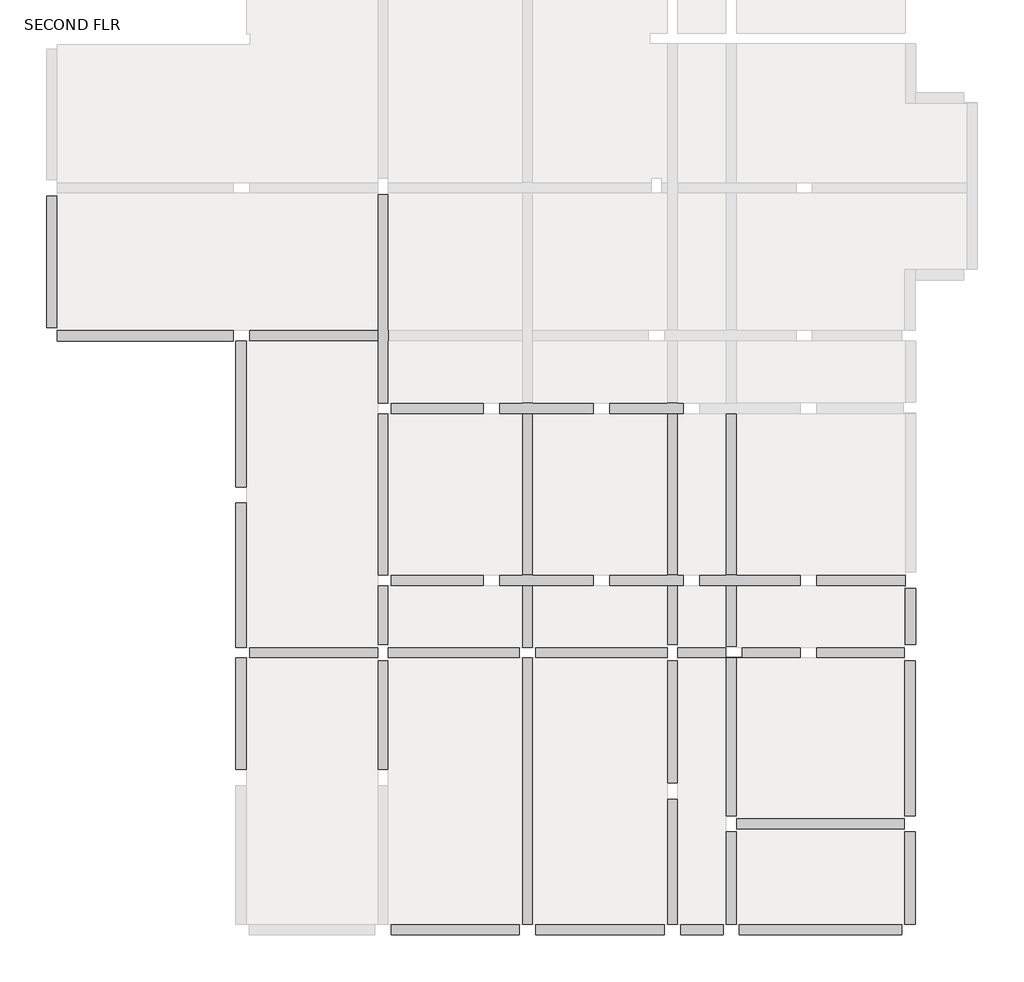
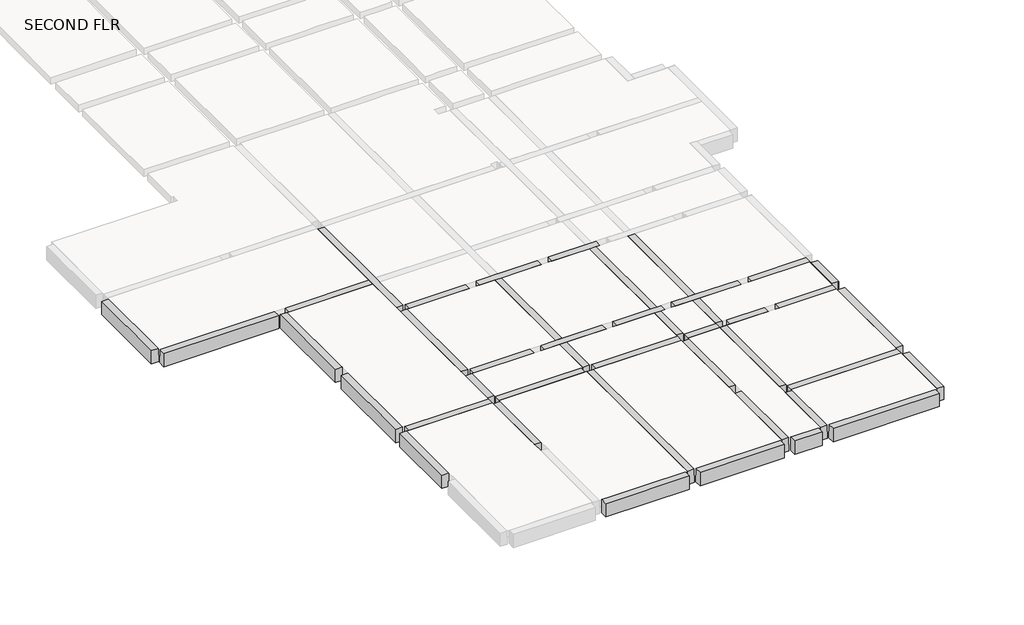
# One storey, part 2 of 4: 42 beams.
"""IFC4 building model written with IfcOpenShell, lengths in millimetres."""

from ifc_helpers import new_model, si_unit, frame, origin, place, context, project, spatial, polyline, outline, extrude, faceted_brep, element, save

model = new_model("IFC4")

# Units and contexts
model_context = context("Model", 3, world=origin())
ifc_project = project(units=[si_unit("LENGTHUNIT", "METRE", prefix="MILLI")], contexts=[model_context])

# Site, building, storey
site = spatial("IfcSite", under=ifc_project)
building = spatial("IfcBuilding", under=site)
storey = spatial("IfcBuildingStorey", under=building, Name="SECOND FLR", Elevation=6048.0)

# Beams
placement = place(None, origin())
element("IfcBeam", 1, ObjectType="M_Concrete-Rectangular Beam : 300 x 600mm", at=placement, inside=storey, context=model_context, shape_type="SweptSolid", body=[
    extrude(outline(polyline([(-10828.8105653, -2764.4535766), (-11128.8105653, -2764.4535766), (-11128.8105653, 876.1713929), (-10828.8105653, 876.1713929), (-10828.8105653, -2764.4535766)])), frame((0.0, 0.0, 5448.0), z_axis=(0.0, 0.0, 1.0), x_axis=(1.0, 0.0, 0.0)), (0.0, 0.0, 1.0), 600.0),
])
element("IfcBeam", 2, ObjectType="M_Concrete-Rectangular Beam : 300 x 600mm", at=placement, inside=storey, context=model_context, shape_type="Brep", body=[
    faceted_brep([(-5963.8105653, -3139.4535766, 6048.0), (-5963.8105653, -2839.4535766, 6048.0), (-10828.8105653, -2839.4535766, 6048.0), (-10828.8105653, -3139.4535766, 6048.0), (-5963.8105653, -3139.4535766, 5448.0), (-10828.8105653, -3139.4535766, 5448.0), (-5963.8105653, -2839.4535766, 5448.0), (-10828.8105653, -2839.4535766, 5448.0), (-5963.8105653, -2839.4535766, 5748.0), (-10828.8105653, -2839.4535766, 5748.0)], [[[0, 1, 2, 3]], [[4, 0, 3, 5]], [[6, 4, 5, 7]], [[2, 1, 8, 6, 7, 9]], [[1, 0, 4, 6, 8]], [[3, 2, 9, 7, 5]]]),
])
element("IfcBeam", 3, ObjectType="M_Concrete-Rectangular Beam : 300 x 600mm", at=placement, inside=storey, context=model_context, shape_type="Brep", body=[
    faceted_brep([(-5588.8105653, -7169.0760584, 6048.0), (-5588.8105653, -3139.4535766, 6048.0), (-5888.8105653, -3139.4535766, 6048.0), (-5888.8105653, -7169.0760584, 6048.0), (-5888.8105653, -3139.4535766, 5448.0), (-5888.8105653, -7169.0760584, 5448.0), (-5588.8105653, -3139.4535766, 5448.0), (-5588.8105653, -7169.0760584, 5448.0), (-5588.8105653, -7169.0760584, 5748.0), (-5588.8105653, -3139.4535766, 5748.0)], [[[0, 1, 2, 3]], [[3, 2, 4, 5]], [[5, 4, 6, 7]], [[1, 0, 8, 7, 6, 9]], [[6, 4, 2, 1, 9]], [[0, 3, 5, 7, 8]]]),
])
element("IfcBeam", 4, ObjectType="M_Concrete-Rectangular Beam : 300 x 600mm", at=placement, inside=storey, context=model_context, shape_type="Brep", body=[
    faceted_brep([(-5588.8105653, -11607.8970059, 6048.0), (-5588.8105653, -7619.0760584, 6048.0), (-5888.8105653, -7619.0760584, 6048.0), (-5888.8105653, -11607.8970059, 6048.0), (-5888.8105653, -7619.0760584, 5448.0), (-5888.8105653, -11607.8970059, 5448.0), (-5588.8105653, -7619.0760584, 5448.0), (-5588.8105653, -11607.8970059, 5448.0), (-5588.8105653, -11607.8970059, 5748.0), (-5588.8105653, -7619.0760584, 5748.0)], [[[0, 1, 2, 3]], [[3, 2, 4, 5]], [[5, 4, 6, 7]], [[1, 0, 8, 7, 6, 9]], [[0, 3, 5, 7, 8]], [[6, 4, 2, 1, 9]]]),
])
element("IfcBeam", 5, ObjectType="M_Concrete-Rectangular Beam : 300 x 600mm", at=placement, inside=storey, context=model_context, shape_type="Brep", body=[
    faceted_brep([(-5588.8105653, -14991.2517597, 6048.0), (-5588.8105653, -11907.8970059, 6048.0), (-5888.8105653, -11907.8970059, 6048.0), (-5888.8105653, -14991.2517597, 6048.0), (-5888.8105653, -11907.8970059, 5448.0), (-5888.8105653, -14991.2517597, 5448.0), (-5588.8105653, -11907.8970059, 5448.0), (-5588.8105653, -14991.2517597, 5448.0), (-5588.8105653, -14991.2517597, 5748.0), (-5588.8105653, -11907.8970059, 5748.0)], [[[0, 1, 2, 3]], [[3, 2, 4, 5]], [[5, 4, 6, 7]], [[1, 0, 8, 7, 6, 9]], [[6, 4, 2, 1, 9]], [[0, 3, 5, 7, 8]]]),
])
element("IfcBeam", 6, ObjectType="M_Concrete-Rectangular Beam : 300 x 600mm", at=placement, inside=storey, context=model_context, shape_type="SweptSolid", body=[
    extrude(outline(polyline([(1949.7296816, -19272.5304373), (1949.7296816, -19572.5304373), (-1596.7865686, -19572.5304373), (-1596.7865686, -19272.5304373), (1949.7296816, -19272.5304373)])), frame((0.0, 0.0, 5448.0), z_axis=(0.0, 0.0, 1.0), x_axis=(1.0, 0.0, 0.0)), (0.0, 0.0, 1.0), 600.0),
])
element("IfcBeam", 7, ObjectType="M_Concrete-Rectangular Beam : 300 x 600mm", at=placement, inside=storey, context=model_context, shape_type="SweptSolid", body=[
    extrude(outline(polyline([(5957.5248054, -19272.5304373), (5957.5248054, -19572.5304373), (2399.7296816, -19572.5304373), (2399.7296816, -19272.5304373), (5957.5248054, -19272.5304373)])), frame((0.0, 0.0, 5448.0), z_axis=(0.0, 0.0, 1.0), x_axis=(1.0, 0.0, 0.0)), (0.0, 0.0, 1.0), 600.0),
])
element("IfcBeam", 8, ObjectType="M_Concrete-Rectangular Beam : 300 x 600mm", at=placement, inside=storey, context=model_context, shape_type="SweptSolid", body=[
    extrude(outline(polyline([(7581.8679014, -19272.5304373), (7581.8679014, -19572.5304373), (6407.5248054, -19572.5304373), (6407.5248054, -19272.5304373), (7581.8679014, -19272.5304373)])), frame((0.0, 0.0, 5448.0), z_axis=(0.0, 0.0, 1.0), x_axis=(1.0, 0.0, 0.0)), (0.0, 0.0, 1.0), 600.0),
])
element("IfcBeam", 9, ObjectType="M_Concrete-Rectangular Beam : 300 x 600mm", at=placement, inside=storey, context=model_context, shape_type="SweptSolid", body=[
    extrude(outline(polyline([(12524.1163908, -19272.5304373), (12524.1163908, -19572.5304373), (8031.8679014, -19572.5304373), (8031.8679014, -19272.5304373), (12524.1163908, -19272.5304373)])), frame((0.0, 0.0, 5448.0), z_axis=(0.0, 0.0, 1.0), x_axis=(1.0, 0.0, 0.0)), (0.0, 0.0, 1.0), 600.0),
])
element("IfcBeam", 10, ObjectType="M_Concrete-Rectangular Beam : 300 x 600mm", at=placement, inside=storey, context=model_context, shape_type="Brep", body=[
    faceted_brep([(12599.1163908, -19272.5304373, 6048.0), (12899.1163908, -19272.5304373, 6048.0), (12899.1163908, -16719.1579597, 6048.0), (12599.1163908, -16719.1579597, 6048.0), (12899.1163908, -19272.5304373, 5448.0), (12899.1163908, -16719.1579597, 5448.0), (12599.1163908, -19272.5304373, 5448.0), (12599.1163908, -16719.1579597, 5448.0), (12599.1163908, -16719.1579597, 5748.0), (12599.1163908, -19272.5304373, 5748.0)], [[[0, 1, 2, 3]], [[1, 4, 5, 2]], [[4, 6, 7, 5]], [[0, 3, 8, 7, 6, 9]], [[6, 4, 1, 0, 9]], [[3, 2, 5, 7, 8]]]),
])
element("IfcBeam", 11, ObjectType="M_Concrete-Rectangular Beam : 300 x 600mm", at=placement, inside=storey, context=model_context, shape_type="Brep", body=[
    faceted_brep([(12599.1163908, -16269.1579597, 6048.0), (12899.1163908, -16269.1579597, 6048.0), (12899.1163908, -11982.8970059, 6048.0), (12599.1163908, -11982.8970059, 6048.0), (12899.1163908, -16269.1579597, 5448.0), (12899.1163908, -11982.8970059, 5448.0), (12599.1163908, -16269.1579597, 5448.0), (12599.1163908, -11982.8970059, 5448.0), (12599.1163908, -11982.8970059, 5748.0), (12599.1163908, -16269.1579597, 5748.0)], [[[0, 1, 2, 3]], [[1, 4, 5, 2]], [[4, 6, 7, 5]], [[0, 3, 8, 7, 6, 9]], [[6, 4, 1, 0, 9]], [[3, 2, 5, 7, 8]]]),
])
element("IfcBeam", 12, ObjectType="M_Concrete-Rectangular Beam : 300 x 600mm", at=placement, inside=storey, context=model_context, shape_type="SweptSolid", body=[
    extrude(outline(polyline([(12619.1163908, -9982.1078267), (12919.1163908, -9982.1078267), (12919.1163908, -11537.8970059), (12899.1163908, -11537.8970059), (12899.1163908, -11532.8970059), (12619.1163908, -11532.8970059), (12619.1163908, -9982.1078267)])), frame((0.0, 0.0, 5448.0), z_axis=(0.0, 0.0, 1.0), x_axis=(1.0, 0.0, 0.0)), (0.0, 0.0, 1.0), 600.0),
])
element("IfcBeam", 13, ObjectType="M_Concrete-Rectangular Beam : 300 x 600mm", at=placement, inside=storey, context=model_context, shape_type="Brep", body=[
    faceted_brep([(-1971.7865686, -11982.8970059, 6048.0), (-1971.7865686, -14991.2517597, 6048.0), (-1671.7865686, -14991.2517597, 6048.0), (-1671.7865686, -11982.8970059, 6048.0), (-1671.7865686, -14991.2517597, 5748.0), (-1671.7865686, -14991.2517597, 5448.0), (-1671.7865686, -11982.8970059, 5448.0), (-1671.7865686, -11982.8970059, 5748.0), (-1971.7865686, -14991.2517597, 5448.0), (-1971.7865686, -11982.8970059, 5448.0), (-1971.7865686, -11982.8970059, 5748.0), (-1971.7865686, -14991.2517597, 5748.0)], [[[0, 1, 2, 3]], [[3, 2, 4, 5, 6, 7]], [[6, 5, 8, 9]], [[1, 0, 10, 9, 8, 11]], [[0, 3, 7, 6, 9, 10]], [[8, 5, 4, 2, 1, 11]]]),
])
element("IfcBeam", 14, ObjectType="M_Concrete-Rectangular Beam : 300 x 600mm", at=placement, inside=storey, context=model_context, shape_type="Brep", body=[
    faceted_brep([(-1971.7865686, -9907.1078267, 6048.0), (-1971.7865686, -11532.8970059, 6048.0), (-1671.7865686, -11532.8970059, 6048.0), (-1671.7865686, -9907.1078267, 6048.0), (-1671.7865686, -11532.8970059, 5748.0), (-1671.7865686, -11532.8970059, 5448.0), (-1671.7865686, -9907.1078267, 5448.0), (-1671.7865686, -9907.1078267, 5748.0), (-1971.7865686, -11532.8970059, 5448.0), (-1971.7865686, -9907.1078267, 5448.0), (-1971.7865686, -9907.1078267, 5748.0), (-1971.7865686, -11532.8970059, 5748.0)], [[[0, 1, 2, 3]], [[3, 2, 4, 5, 6, 7]], [[6, 5, 8, 9]], [[1, 0, 10, 9, 8, 11]], [[0, 3, 7, 6, 9, 10]], [[8, 5, 4, 2, 1, 11]]]),
])
element("IfcBeam", 15, ObjectType="M_Concrete-Rectangular Beam : 300 x 600mm", at=placement, inside=storey, context=model_context, shape_type="Brep", body=[
    faceted_brep([(-1671.7865686, 916.1713929, 6048.0), (-1971.7865686, 916.1713929, 6048.0), (-1971.7865686, -2839.4535766, 6048.0), (-1971.7865686, -3139.4535766, 6048.0), (-1971.7865686, -4851.6229916, 6048.0), (-1671.7865686, -4851.6229916, 6048.0), (-1671.7865686, -3139.4535766, 6048.0), (-1671.7865686, -2839.4535766, 6048.0), (-1971.7865686, 916.1713929, 5448.0), (-1971.7865686, -2839.4535766, 5448.0), (-1971.7865686, -3139.4535766, 5448.0), (-1971.7865686, -4851.6229916, 5448.0), (-1971.7865686, -4851.6229916, 5748.0), (-1971.7865686, 916.1713929, 5748.0), (-1671.7865686, 916.1713929, 5448.0), (-1671.7865686, -2839.4535766, 5448.0), (-1671.7865686, -3139.4535766, 5448.0), (-1671.7865686, -4851.6229916, 5448.0), (-1671.7865686, 916.1713929, 5748.0), (-1671.7865686, -4851.6229916, 5748.0)], [[[0, 1, 2, 3, 4, 5, 6, 7]], [[8, 9, 10, 11, 12, 4, 3, 2, 1, 13]], [[8, 14, 15, 16, 17, 11, 10, 9]], [[17, 16, 15, 14, 18, 0, 7, 6, 5, 19]], [[1, 0, 18, 14, 8, 13]], [[5, 4, 12, 11, 17, 19]]]),
])
element("IfcBeam", 16, ObjectType="M_Concrete-Rectangular Beam : 300 x 600mm", at=placement, inside=storey, context=model_context, shape_type="Brep", body=[
    faceted_brep([(-1671.7865686, -5151.6229916, 6048.0), (-1971.7865686, -5151.6229916, 6048.0), (-1971.7865686, -9607.1078267, 6048.0), (-1671.7865686, -9607.1078267, 6048.0), (-1971.7865686, -5151.6229916, 5748.0), (-1971.7865686, -5151.6229916, 5448.0), (-1971.7865686, -9607.1078267, 5448.0), (-1971.7865686, -9607.1078267, 5748.0), (-1671.7865686, -5151.6229916, 5448.0), (-1671.7865686, -9607.1078267, 5448.0), (-1671.7865686, -9607.1078267, 5748.0), (-1671.7865686, -5151.6229916, 5748.0)], [[[0, 1, 2, 3]], [[2, 1, 4, 5, 6, 7]], [[5, 8, 9, 6]], [[0, 3, 10, 9, 8, 11]], [[1, 0, 11, 8, 5, 4]], [[3, 2, 7, 6, 9, 10]]]),
])
element("IfcBeam", 17, ObjectType="M_Concrete-Rectangular Beam : 300 x 600mm", at=placement, inside=storey, context=model_context, shape_type="Brep", body=[
    faceted_brep([(2324.7296816, -11907.8970059, 6048.0), (2024.7296816, -11907.8970059, 6048.0), (2024.7296816, -19272.5304373, 6048.0), (2324.7296816, -19272.5304373, 6048.0), (2024.7296816, -11907.8970059, 5748.0), (2024.7296816, -11907.8970059, 5448.0), (2024.7296816, -19272.5304373, 5448.0), (2024.7296816, -19272.5304373, 5748.0), (2324.7296816, -11907.8970059, 5448.0), (2324.7296816, -19272.5304373, 5448.0), (2324.7296816, -19272.5304373, 5748.0), (2324.7296816, -11907.8970059, 5748.0)], [[[0, 1, 2, 3]], [[2, 1, 4, 5, 6, 7]], [[5, 8, 9, 6]], [[0, 3, 10, 9, 8, 11]], [[1, 0, 11, 8, 5, 4]], [[3, 2, 7, 6, 9, 10]]]),
])
element("IfcBeam", 18, ObjectType="M_Concrete-Rectangular Beam : 300 x 600mm", at=placement, inside=storey, context=model_context, shape_type="Brep", body=[
    faceted_brep([(6332.5248054, -11982.8970059, 6048.0), (6032.5248054, -11982.8970059, 6048.0), (6032.5248054, -15369.1579597, 6048.0), (6332.5248054, -15369.1579597, 6048.0), (6032.5248054, -11982.8970059, 5748.0), (6032.5248054, -11982.8970059, 5448.0), (6032.5248054, -15369.1579597, 5448.0), (6032.5248054, -15369.1579597, 5748.0), (6332.5248054, -11982.8970059, 5448.0), (6332.5248054, -15369.1579597, 5448.0), (6332.5248054, -15369.1579597, 5748.0), (6332.5248054, -11982.8970059, 5748.0)], [[[0, 1, 2, 3]], [[2, 1, 4, 5, 6, 7]], [[5, 8, 9, 6]], [[0, 3, 10, 9, 8, 11]], [[1, 0, 11, 8, 5, 4]], [[3, 2, 7, 6, 9, 10]]]),
])
element("IfcBeam", 19, ObjectType="M_Concrete-Rectangular Beam : 300 x 600mm", at=placement, inside=storey, context=model_context, shape_type="Brep", body=[
    faceted_brep([(6032.5248054, -19272.5304373, 6048.0), (6332.5248054, -19272.5304373, 6048.0), (6332.5248054, -15819.1579597, 6048.0), (6032.5248054, -15819.1579597, 6048.0), (6032.5248054, -15819.1579597, 5748.0), (6032.5248054, -15819.1579597, 5448.0), (6032.5248054, -19272.5304373, 5448.0), (6032.5248054, -19272.5304373, 5748.0), (6332.5248054, -19272.5304373, 5448.0), (6332.5248054, -15819.1579597, 5448.0), (6332.5248054, -19272.5304373, 5748.0), (6332.5248054, -15819.1579597, 5748.0)], [[[0, 1, 2, 3]], [[0, 3, 4, 5, 6, 7]], [[8, 6, 5, 9]], [[2, 1, 10, 8, 9, 11]], [[1, 0, 7, 6, 8, 10]], [[3, 2, 11, 9, 5, 4]]]),
])
element("IfcBeam", 20, ObjectType="M_Concrete-Rectangular Beam : 300 x 600mm", at=placement, inside=storey, context=model_context, shape_type="Brep", body=[
    faceted_brep([(7656.8679014, -19272.5304373, 6048.0), (7956.8679014, -19272.5304373, 6048.0), (7956.8679014, -16719.1579597, 6048.0), (7656.8679014, -16719.1579597, 6048.0), (7656.8679014, -16719.1579597, 5748.0), (7656.8679014, -16719.1579597, 5448.0), (7656.8679014, -19272.5304373, 5448.0), (7656.8679014, -19272.5304373, 5748.0), (7956.8679014, -19272.5304373, 5448.0), (7956.8679014, -16719.1579597, 5448.0), (7956.8679014, -19272.5304373, 5748.0), (7956.8679014, -16719.1579597, 5748.0)], [[[0, 1, 2, 3]], [[0, 3, 4, 5, 6, 7]], [[8, 6, 5, 9]], [[2, 1, 10, 8, 9, 11]], [[1, 0, 7, 6, 8, 10]], [[3, 2, 11, 9, 5, 4]]]),
])
element("IfcBeam", 21, ObjectType="M_Concrete-Rectangular Beam : 300 x 600mm", at=placement, inside=storey, context=model_context, shape_type="Brep", body=[
    faceted_brep([(-5513.8105653, -2839.4535766, 6048.0), (-5513.8105653, -3139.4535766, 6048.0), (-1971.7865686, -3139.4535766, 6048.0), (-1971.7865686, -2839.4535766, 6048.0), (-5513.8105653, -3139.4535766, 5748.0), (-5513.8105653, -3139.4535766, 5448.0), (-1971.7865686, -3139.4535766, 5448.0), (-1971.7865686, -3139.4535766, 5748.0), (-5513.8105653, -2839.4535766, 5448.0), (-1971.7865686, -2839.4535766, 5448.0), (-1971.7865686, -2839.4535766, 5748.0), (-5513.8105653, -2839.4535766, 5748.0)], [[[0, 1, 2, 3]], [[2, 1, 4, 5, 6, 7]], [[5, 8, 9, 6]], [[0, 3, 10, 9, 8, 11]], [[1, 0, 11, 8, 5, 4]], [[3, 2, 7, 6, 9, 10]]]),
])
element("IfcBeam", 22, ObjectType="M_Concrete-Rectangular Beam : 300 x 600mm", at=placement, inside=storey, context=model_context, shape_type="Brep", body=[
    faceted_brep([(-1596.7865686, -4851.6229916, 6048.0), (-1596.7865686, -5151.6229916, 6048.0), (949.7296816, -5151.6229916, 6048.0), (949.7296816, -4851.6229916, 6048.0), (-1596.7865686, -5151.6229916, 5748.0), (-1596.7865686, -5151.6229916, 5448.0), (949.7296816, -5151.6229916, 5448.0), (949.7296816, -5151.6229916, 5748.0), (-1596.7865686, -4851.6229916, 5448.0), (949.7296816, -4851.6229916, 5448.0), (949.7296816, -4851.6229916, 5748.0), (-1596.7865686, -4851.6229916, 5748.0)], [[[0, 1, 2, 3]], [[2, 1, 4, 5, 6, 7]], [[5, 8, 9, 6]], [[0, 3, 10, 9, 8, 11]], [[1, 0, 11, 8, 5, 4]], [[3, 2, 7, 6, 9, 10]]]),
])
element("IfcBeam", 23, ObjectType="M_Concrete-Rectangular Beam : 300 x 600mm", at=placement, inside=storey, context=model_context, shape_type="Brep", body=[
    faceted_brep([(1399.7296816, -4851.6229916, 6048.0), (1399.7296816, -5151.6229916, 6048.0), (2024.7296816, -5151.6229916, 6048.0), (2324.7296816, -5151.6229916, 6048.0), (3997.5248054, -5151.6229916, 6048.0), (3997.5248054, -4851.6229916, 6048.0), (2324.7296816, -4851.6229916, 6048.0), (2024.7296816, -4851.6229916, 6048.0), (1399.7296816, -5151.6229916, 5448.0), (2024.7296816, -5151.6229916, 5448.0), (2324.7296816, -5151.6229916, 5448.0), (3997.5248054, -5151.6229916, 5448.0), (3997.5248054, -5151.6229916, 5748.0), (1399.7296816, -5151.6229916, 5748.0), (1399.7296816, -4851.6229916, 5448.0), (2024.7296816, -4851.6229916, 5448.0), (2324.7296816, -4851.6229916, 5448.0), (3997.5248054, -4851.6229916, 5448.0), (1399.7296816, -4851.6229916, 5748.0), (3997.5248054, -4851.6229916, 5748.0)], [[[0, 1, 2, 3, 4, 5, 6, 7]], [[8, 9, 10, 11, 12, 4, 3, 2, 1, 13]], [[8, 14, 15, 16, 17, 11, 10, 9]], [[17, 16, 15, 14, 18, 0, 7, 6, 5, 19]], [[1, 0, 18, 14, 8, 13]], [[5, 4, 12, 11, 17, 19]]]),
])
element("IfcBeam", 24, ObjectType="M_Concrete-Rectangular Beam : 300 x 600mm", at=placement, inside=storey, context=model_context, shape_type="Brep", body=[
    faceted_brep([(4447.5248054, -4851.6229916, 6048.0), (4447.5248054, -5151.6229916, 6048.0), (6032.5248054, -5151.6229916, 6048.0), (6332.5248054, -5151.6229916, 6048.0), (6481.8679014, -5151.6229916, 6048.0), (6481.8679014, -4851.6229916, 6048.0), (6332.5248054, -4851.6229916, 6048.0), (6032.5248054, -4851.6229916, 6048.0), (4447.5248054, -5151.6229916, 5448.0), (6032.5248054, -5151.6229916, 5448.0), (6332.5248054, -5151.6229916, 5448.0), (6481.8679014, -5151.6229916, 5448.0), (6481.8679014, -5151.6229916, 5748.0), (4447.5248054, -5151.6229916, 5748.0), (4447.5248054, -4851.6229916, 5448.0), (6032.5248054, -4851.6229916, 5448.0), (6332.5248054, -4851.6229916, 5448.0), (6481.8679014, -4851.6229916, 5448.0), (4447.5248054, -4851.6229916, 5748.0)], [[[0, 1, 2, 3, 4, 5, 6, 7]], [[8, 9, 10, 11, 12, 4, 3, 2, 1, 13]], [[8, 14, 15, 16, 17, 11, 10, 9]], [[17, 16, 15, 14, 18, 0, 7, 6, 5]], [[1, 0, 18, 14, 8, 13]], [[5, 4, 12, 11, 17]]]),
])
element("IfcBeam", 25, ObjectType="M_Concrete-Rectangular Beam : 300 x 600mm", at=placement, inside=storey, context=model_context, shape_type="Brep", body=[
    faceted_brep([(-1971.7865686, -11907.8970059, 6048.0), (-1971.7865686, -11607.8970059, 6048.0), (-5513.8105653, -11607.8970059, 6048.0), (-5513.8105653, -11907.8970059, 6048.0), (-5513.8105653, -11907.8970059, 5748.0), (-5513.8105653, -11907.8970059, 5448.0), (-1971.7865686, -11907.8970059, 5448.0), (-1971.7865686, -11907.8970059, 5748.0), (-1971.7865686, -11607.8970059, 5448.0), (-5513.8105653, -11607.8970059, 5448.0), (-1971.7865686, -11607.8970059, 5748.0), (-5513.8105653, -11607.8970059, 5748.0)], [[[0, 1, 2, 3]], [[0, 3, 4, 5, 6, 7]], [[8, 6, 5, 9]], [[2, 1, 10, 8, 9, 11]], [[1, 0, 7, 6, 8, 10]], [[3, 2, 11, 9, 5, 4]]]),
])
element("IfcBeam", 26, ObjectType="M_Concrete-Rectangular Beam : 300 x 600mm", at=placement, inside=storey, context=model_context, shape_type="Brep", body=[
    faceted_brep([(1949.7296816, -11907.8970059, 6048.0), (1949.7296816, -11607.8970059, 6048.0), (-1671.7865686, -11607.8970059, 6048.0), (-1671.7865686, -11907.8970059, 6048.0), (-1671.7865686, -11907.8970059, 5748.0), (-1671.7865686, -11907.8970059, 5448.0), (1949.7296816, -11907.8970059, 5448.0), (1949.7296816, -11907.8970059, 5748.0), (1949.7296816, -11607.8970059, 5448.0), (-1671.7865686, -11607.8970059, 5448.0), (1949.7296816, -11607.8970059, 5748.0), (-1671.7865686, -11607.8970059, 5748.0)], [[[0, 1, 2, 3]], [[0, 3, 4, 5, 6, 7]], [[8, 6, 5, 9]], [[2, 1, 10, 8, 9, 11]], [[1, 0, 7, 6, 8, 10]], [[3, 2, 11, 9, 5, 4]]]),
])
element("IfcBeam", 27, ObjectType="M_Concrete-Rectangular Beam : 300 x 600mm", at=placement, inside=storey, context=model_context, shape_type="Brep", body=[
    faceted_brep([(6032.5248054, -11907.8970059, 6048.0), (6032.5248054, -11607.8970059, 6048.0), (2399.7296816, -11607.8970059, 6048.0), (2399.7296816, -11907.8970059, 6048.0), (2399.7296816, -11907.8970059, 5748.0), (2399.7296816, -11907.8970059, 5448.0), (6032.5248054, -11907.8970059, 5448.0), (6032.5248054, -11907.8970059, 5748.0), (6032.5248054, -11607.8970059, 5448.0), (2399.7296816, -11607.8970059, 5448.0), (6032.5248054, -11607.8970059, 5748.0), (2399.7296816, -11607.8970059, 5748.0)], [[[0, 1, 2, 3]], [[0, 3, 4, 5, 6, 7]], [[8, 6, 5, 9]], [[2, 1, 10, 8, 9, 11]], [[1, 0, 7, 6, 8, 10]], [[3, 2, 11, 9, 5, 4]]]),
])
element("IfcBeam", 28, ObjectType="M_Concrete-Rectangular Beam : 300 x 600mm", at=placement, inside=storey, context=model_context, shape_type="Brep", body=[
    faceted_brep([(9721.8679014, -11907.8970059, 6048.0), (9721.8679014, -11607.8970059, 6048.0), (8111.8679014, -11607.8970059, 6048.0), (8111.8679014, -11887.8970059, 6048.0), (7661.8679014, -11887.8970059, 6048.0), (7661.8679014, -11607.8970059, 6048.0), (7656.8679014, -11607.8970059, 6048.0), (6332.5248054, -11607.8970059, 6048.0), (6332.5248054, -11907.8970059, 6048.0), (7656.8679014, -11907.8970059, 6048.0), (7956.8679014, -11907.8970059, 6048.0), (6332.5248054, -11907.8970059, 5448.0), (7656.8679014, -11907.8970059, 5448.0), (7956.8679014, -11907.8970059, 5448.0), (9721.8679014, -11907.8970059, 5448.0), (9721.8679014, -11907.8970059, 5748.0), (6332.5248054, -11907.8970059, 5748.0), (9721.8679014, -11607.8970059, 5448.0), (6332.5248054, -11607.8970059, 5448.0), (7656.8679014, -11607.8970059, 5448.0), (7661.8679014, -11607.8970059, 5448.0), (7661.8679014, -11887.8970059, 5448.0), (8111.8679014, -11887.8970059, 5448.0), (8111.8679014, -11607.8970059, 5448.0), (6332.5248054, -11607.8970059, 5748.0), (9721.8679014, -11607.8970059, 5748.0), (8111.8679014, -11607.8970059, 5748.0)], [[[0, 1, 2, 3, 4, 5, 6, 7, 8, 9, 10]], [[11, 12, 13, 14, 15, 0, 10, 9, 8, 16]], [[17, 14, 13, 12, 11, 18, 19, 20, 21, 22, 23]], [[20, 19, 18, 24, 7, 6, 5]], [[1, 0, 15, 14, 17, 25]], [[8, 7, 24, 18, 11, 16]], [[22, 3, 2, 26, 23]], [[3, 22, 21, 4]], [[4, 21, 20, 5]], [[2, 1, 25, 17, 23, 26]]]),
])
element("IfcBeam", 29, ObjectType="M_Concrete-Rectangular Beam : 300 x 600mm", at=placement, inside=storey, context=model_context, shape_type="Brep", body=[
    faceted_brep([(12599.1163908, -11907.8970059, 6048.0), (12599.1163908, -11607.8970059, 6048.0), (10171.8679014, -11607.8970059, 6048.0), (10171.8679014, -11907.8970059, 6048.0), (10171.8679014, -11907.8970059, 5748.0), (10171.8679014, -11907.8970059, 5448.0), (12599.1163908, -11907.8970059, 5448.0), (12599.1163908, -11907.8970059, 5748.0), (12599.1163908, -11607.8970059, 5448.0), (10171.8679014, -11607.8970059, 5448.0), (12599.1163908, -11607.8970059, 5748.0), (10171.8679014, -11607.8970059, 5748.0)], [[[0, 1, 2, 3]], [[0, 3, 4, 5, 6, 7]], [[8, 6, 5, 9]], [[2, 1, 10, 8, 9, 11]], [[1, 0, 7, 6, 8, 10]], [[3, 2, 11, 9, 5, 4]]]),
])
element("IfcBeam", 30, ObjectType="M_Concrete-Rectangular Beam : 300 x 600mm", at=placement, inside=storey, context=model_context, shape_type="Brep", body=[
    faceted_brep([(12599.1163908, -16644.1579597, 6048.0), (12599.1163908, -16344.1579597, 6048.0), (7956.8679014, -16344.1579597, 6048.0), (7956.8679014, -16644.1579597, 6048.0), (7956.8679014, -16644.1579597, 5748.0), (7956.8679014, -16644.1579597, 5448.0), (12599.1163908, -16644.1579597, 5448.0), (12599.1163908, -16644.1579597, 5748.0), (12599.1163908, -16344.1579597, 5448.0), (7956.8679014, -16344.1579597, 5448.0), (12599.1163908, -16344.1579597, 5748.0), (7956.8679014, -16344.1579597, 5748.0)], [[[0, 1, 2, 3]], [[0, 3, 4, 5, 6, 7]], [[8, 6, 5, 9]], [[2, 1, 10, 8, 9, 11]], [[1, 0, 7, 6, 8, 10]], [[3, 2, 11, 9, 5, 4]]]),
])
element("IfcBeam", 31, ObjectType="M_Concrete-Rectangular Beam : 300 x 600mm", at=placement, inside=storey, context=model_context, shape_type="Brep", body=[
    faceted_brep([(-1596.7865686, -9607.1078267, 6048.0), (-1596.7865686, -9907.1078267, 6048.0), (949.7296816, -9907.1078267, 6048.0), (949.7296816, -9607.1078267, 6048.0), (-1596.7865686, -9907.1078267, 5748.0), (-1596.7865686, -9907.1078267, 5448.0), (949.7296816, -9907.1078267, 5448.0), (949.7296816, -9907.1078267, 5748.0), (-1596.7865686, -9607.1078267, 5448.0), (949.7296816, -9607.1078267, 5448.0), (949.7296816, -9607.1078267, 5748.0), (-1596.7865686, -9607.1078267, 5748.0)], [[[0, 1, 2, 3]], [[2, 1, 4, 5, 6, 7]], [[5, 8, 9, 6]], [[0, 3, 10, 9, 8, 11]], [[1, 0, 11, 8, 5, 4]], [[3, 2, 7, 6, 9, 10]]]),
])
element("IfcBeam", 32, ObjectType="M_Concrete-Rectangular Beam : 300 x 600mm", at=placement, inside=storey, context=model_context, shape_type="Brep", body=[
    faceted_brep([(1399.7296816, -9607.1078267, 6048.0), (1399.7296816, -9907.1078267, 6048.0), (2024.7296816, -9907.1078267, 6048.0), (2324.7296816, -9907.1078267, 6048.0), (3997.5248054, -9907.1078267, 6048.0), (3997.5248054, -9607.1078267, 6048.0), (2324.7296816, -9607.1078267, 6048.0), (2024.7296816, -9607.1078267, 6048.0), (1399.7296816, -9907.1078267, 5448.0), (2024.7296816, -9907.1078267, 5448.0), (2324.7296816, -9907.1078267, 5448.0), (3997.5248054, -9907.1078267, 5448.0), (3997.5248054, -9907.1078267, 5748.0), (1399.7296816, -9907.1078267, 5748.0), (1399.7296816, -9607.1078267, 5448.0), (2024.7296816, -9607.1078267, 5448.0), (2324.7296816, -9607.1078267, 5448.0), (3997.5248054, -9607.1078267, 5448.0), (1399.7296816, -9607.1078267, 5748.0), (3997.5248054, -9607.1078267, 5748.0)], [[[0, 1, 2, 3, 4, 5, 6, 7]], [[8, 9, 10, 11, 12, 4, 3, 2, 1, 13]], [[8, 14, 15, 16, 17, 11, 10, 9]], [[17, 16, 15, 14, 18, 0, 7, 6, 5, 19]], [[1, 0, 18, 14, 8, 13]], [[5, 4, 12, 11, 17, 19]]]),
])
element("IfcBeam", 33, ObjectType="M_Concrete-Rectangular Beam : 300 x 600mm", at=placement, inside=storey, context=model_context, shape_type="Brep", body=[
    faceted_brep([(4447.5248054, -9607.1078267, 6048.0), (4447.5248054, -9907.1078267, 6048.0), (6032.5248054, -9907.1078267, 6048.0), (6332.5248054, -9907.1078267, 6048.0), (6481.8679014, -9907.1078267, 6048.0), (6481.8679014, -9607.1078267, 6048.0), (6332.5248054, -9607.1078267, 6048.0), (6032.5248054, -9607.1078267, 6048.0), (4447.5248054, -9907.1078267, 5448.0), (6032.5248054, -9907.1078267, 5448.0), (6332.5248054, -9907.1078267, 5448.0), (6481.8679014, -9907.1078267, 5448.0), (6481.8679014, -9907.1078267, 5748.0), (4447.5248054, -9907.1078267, 5748.0), (4447.5248054, -9607.1078267, 5448.0), (6032.5248054, -9607.1078267, 5448.0), (6332.5248054, -9607.1078267, 5448.0), (6481.8679014, -9607.1078267, 5448.0), (4447.5248054, -9607.1078267, 5748.0), (6481.8679014, -9607.1078267, 5748.0)], [[[0, 1, 2, 3, 4, 5, 6, 7]], [[8, 9, 10, 11, 12, 4, 3, 2, 1, 13]], [[8, 14, 15, 16, 17, 11, 10, 9]], [[17, 16, 15, 14, 18, 0, 7, 6, 5, 19]], [[1, 0, 18, 14, 8, 13]], [[5, 4, 12, 11, 17, 19]]]),
])
element("IfcBeam", 34, ObjectType="M_Concrete-Rectangular Beam : 300 x 600mm", at=placement, inside=storey, context=model_context, shape_type="Brep", body=[
    faceted_brep([(6931.8679014, -9607.1078267, 6048.0), (6931.8679014, -9907.1078267, 6048.0), (7656.8679014, -9907.1078267, 6048.0), (7956.8679014, -9907.1078267, 6048.0), (9721.8679014, -9907.1078267, 6048.0), (9721.8679014, -9607.1078267, 6048.0), (7956.8679014, -9607.1078267, 6048.0), (7656.8679014, -9607.1078267, 6048.0), (6931.8679014, -9907.1078267, 5448.0), (7656.8679014, -9907.1078267, 5448.0), (7956.8679014, -9907.1078267, 5448.0), (9721.8679014, -9907.1078267, 5448.0), (9721.8679014, -9907.1078267, 5748.0), (6931.8679014, -9907.1078267, 5748.0), (6931.8679014, -9607.1078267, 5448.0), (7656.8679014, -9607.1078267, 5448.0), (7956.8679014, -9607.1078267, 5448.0), (9721.8679014, -9607.1078267, 5448.0), (6931.8679014, -9607.1078267, 5748.0), (9721.8679014, -9607.1078267, 5748.0)], [[[0, 1, 2, 3, 4, 5, 6, 7]], [[8, 9, 10, 11, 12, 4, 3, 2, 1, 13]], [[8, 14, 15, 16, 17, 11, 10, 9]], [[17, 16, 15, 14, 18, 0, 7, 6, 5, 19]], [[1, 0, 18, 14, 8, 13]], [[5, 4, 12, 11, 17, 19]]]),
])
element("IfcBeam", 35, ObjectType="M_Concrete-Rectangular Beam : 300 x 600mm", at=placement, inside=storey, context=model_context, shape_type="Brep", body=[
    faceted_brep([(10171.8679014, -9607.1078267, 6048.0), (10171.8679014, -9907.1078267, 6048.0), (12599.1163908, -9907.1078267, 6048.0), (12619.1163908, -9907.1078267, 6048.0), (12619.1163908, -9607.1078267, 6048.0), (10171.8679014, -9907.1078267, 5448.0), (12619.1163908, -9907.1078267, 5448.0), (10171.8679014, -9907.1078267, 5748.0), (10171.8679014, -9607.1078267, 5448.0), (12619.1163908, -9607.1078267, 5448.0), (12619.1163908, -9607.1078267, 5748.0), (10171.8679014, -9607.1078267, 5748.0)], [[[0, 1, 2, 3, 4]], [[5, 6, 3, 2, 1, 7]], [[5, 8, 9, 6]], [[0, 4, 10, 9, 8, 11]], [[1, 0, 11, 8, 5, 7]], [[4, 3, 6, 9, 10]]]),
])
element("IfcBeam", 36, ObjectType="M_Concrete-Rectangular Beam : 300 x 600mm", at=placement, inside=storey, context=model_context, shape_type="Brep", body=[
    faceted_brep([(2324.7296816, -5151.6229916, 6048.0), (2024.7296816, -5151.6229916, 6048.0), (2024.7296816, -9607.1078267, 6048.0), (2324.7296816, -9607.1078267, 6048.0), (2024.7296816, -5151.6229916, 5748.0), (2024.7296816, -5151.6229916, 5448.0), (2024.7296816, -9607.1078267, 5448.0), (2024.7296816, -9607.1078267, 5748.0), (2324.7296816, -5151.6229916, 5448.0), (2324.7296816, -9607.1078267, 5448.0), (2324.7296816, -9607.1078267, 5748.0), (2324.7296816, -5151.6229916, 5748.0)], [[[0, 1, 2, 3]], [[2, 1, 4, 5, 6, 7]], [[5, 8, 9, 6]], [[0, 3, 10, 9, 8, 11]], [[1, 0, 11, 8, 5, 4]], [[3, 2, 7, 6, 9, 10]]]),
])
element("IfcBeam", 37, ObjectType="M_Concrete-Rectangular Beam : 300 x 600mm", at=placement, inside=storey, context=model_context, shape_type="Brep", body=[
    faceted_brep([(6332.5248054, -5151.6229916, 6048.0), (6032.5248054, -5151.6229916, 6048.0), (6032.5248054, -9607.1078267, 6048.0), (6332.5248054, -9607.1078267, 6048.0), (6032.5248054, -5151.6229916, 5748.0), (6032.5248054, -5151.6229916, 5448.0), (6032.5248054, -9607.1078267, 5448.0), (6032.5248054, -9607.1078267, 5748.0), (6332.5248054, -5151.6229916, 5448.0), (6332.5248054, -9607.1078267, 5448.0), (6332.5248054, -9607.1078267, 5748.0), (6332.5248054, -5151.6229916, 5748.0)], [[[0, 1, 2, 3]], [[2, 1, 4, 5, 6, 7]], [[5, 8, 9, 6]], [[0, 3, 10, 9, 8, 11]], [[1, 0, 11, 8, 5, 4]], [[3, 2, 7, 6, 9, 10]]]),
])
element("IfcBeam", 38, ObjectType="M_Concrete-Rectangular Beam : 300 x 600mm", at=placement, inside=storey, context=model_context, shape_type="Brep", body=[
    faceted_brep([(7956.8679014, -5151.6229916, 6048.0), (7656.8679014, -5151.6229916, 6048.0), (7656.8679014, -9607.1078267, 6048.0), (7956.8679014, -9607.1078267, 6048.0), (7656.8679014, -5151.6229916, 5748.0), (7656.8679014, -5151.6229916, 5448.0), (7656.8679014, -9607.1078267, 5448.0), (7656.8679014, -9607.1078267, 5748.0), (7956.8679014, -5151.6229916, 5448.0), (7956.8679014, -9607.1078267, 5448.0), (7956.8679014, -9607.1078267, 5748.0), (7956.8679014, -5151.6229916, 5748.0)], [[[0, 1, 2, 3]], [[2, 1, 4, 5, 6, 7]], [[5, 8, 9, 6]], [[0, 3, 10, 9, 8, 11]], [[1, 0, 11, 8, 5, 4]], [[3, 2, 7, 6, 9, 10]]]),
])
element("IfcBeam", 39, ObjectType="M_Concrete-Rectangular Beam : 300 x 600mm", at=placement, inside=storey, context=model_context, shape_type="Brep", body=[
    faceted_brep([(7656.8679014, -16269.1579597, 6048.0), (7956.8679014, -16269.1579597, 6048.0), (7956.8679014, -11907.8970059, 6048.0), (7656.8679014, -11907.8970059, 6048.0), (7656.8679014, -11907.8970059, 5748.0), (7656.8679014, -11907.8970059, 5448.0), (7656.8679014, -16269.1579597, 5448.0), (7656.8679014, -16269.1579597, 5748.0), (7956.8679014, -16269.1579597, 5448.0), (7956.8679014, -11907.8970059, 5448.0), (7956.8679014, -16269.1579597, 5748.0), (7956.8679014, -11907.8970059, 5748.0)], [[[0, 1, 2, 3]], [[0, 3, 4, 5, 6, 7]], [[8, 6, 5, 9]], [[2, 1, 10, 8, 9, 11]], [[1, 0, 7, 6, 8, 10]], [[3, 2, 11, 9, 5, 4]]]),
])
element("IfcBeam", 40, ObjectType="M_Concrete-Rectangular Beam : 300 x 600mm", at=placement, inside=storey, context=model_context, shape_type="Brep", body=[
    faceted_brep([(2024.7296816, -11607.8970059, 6048.0), (2324.7296816, -11607.8970059, 6048.0), (2324.7296816, -9907.1078267, 6048.0), (2024.7296816, -9907.1078267, 6048.0), (2024.7296816, -9907.1078267, 5748.0), (2024.7296816, -9907.1078267, 5448.0), (2024.7296816, -11607.8970059, 5448.0), (2024.7296816, -11607.8970059, 5748.0), (2324.7296816, -11607.8970059, 5448.0), (2324.7296816, -9907.1078267, 5448.0), (2324.7296816, -11607.8970059, 5748.0), (2324.7296816, -9907.1078267, 5748.0)], [[[0, 1, 2, 3]], [[0, 3, 4, 5, 6, 7]], [[8, 6, 5, 9]], [[2, 1, 10, 8, 9, 11]], [[1, 0, 7, 6, 8, 10]], [[3, 2, 11, 9, 5, 4]]]),
])
element("IfcBeam", 41, ObjectType="M_Concrete-Rectangular Beam : 300 x 600mm", at=placement, inside=storey, context=model_context, shape_type="Brep", body=[
    faceted_brep([(6032.5248054, -11532.8970059, 6048.0), (6332.5248054, -11532.8970059, 6048.0), (6332.5248054, -9907.1078267, 6048.0), (6032.5248054, -9907.1078267, 6048.0), (6032.5248054, -9907.1078267, 5748.0), (6032.5248054, -9907.1078267, 5448.0), (6032.5248054, -11532.8970059, 5448.0), (6032.5248054, -11532.8970059, 5748.0), (6332.5248054, -11532.8970059, 5448.0), (6332.5248054, -9907.1078267, 5448.0), (6332.5248054, -11532.8970059, 5748.0), (6332.5248054, -9907.1078267, 5748.0)], [[[0, 1, 2, 3]], [[0, 3, 4, 5, 6, 7]], [[8, 6, 5, 9]], [[2, 1, 10, 8, 9, 11]], [[1, 0, 7, 6, 8, 10]], [[3, 2, 11, 9, 5, 4]]]),
])
element("IfcBeam", 42, ObjectType="M_Concrete-Rectangular Beam : 300 x 600mm", at=placement, inside=storey, context=model_context, shape_type="Brep", body=[
    faceted_brep([(7661.8679014, -11587.8970059, 6048.0), (7956.8679014, -11587.8970059, 6048.0), (7956.8679014, -9907.1078267, 6048.0), (7656.8679014, -9907.1078267, 6048.0), (7656.8679014, -11607.8970059, 6048.0), (7661.8679014, -11607.8970059, 6048.0), (7656.8679014, -9907.1078267, 5748.0), (7656.8679014, -9907.1078267, 5448.0), (7656.8679014, -11607.8970059, 5448.0), (7656.8679014, -11607.8970059, 5748.0), (7956.8679014, -11587.8970059, 5448.0), (7661.8679014, -11587.8970059, 5448.0), (7661.8679014, -11607.8970059, 5448.0), (7956.8679014, -9907.1078267, 5448.0), (7956.8679014, -11587.8970059, 5748.0), (7956.8679014, -9907.1078267, 5748.0)], [[[0, 1, 2, 3, 4, 5]], [[4, 3, 6, 7, 8, 9]], [[10, 11, 12, 8, 7, 13]], [[2, 1, 14, 10, 13, 15]], [[0, 11, 10, 14, 1]], [[11, 0, 5, 12]], [[3, 2, 15, 13, 7, 6]], [[5, 4, 9, 8, 12]]]),
])

save(model, "model.ifc")

# Revit data of these elements
# Type "M_Concrete-Rectangular Beam : 300 x 600mm"
#   Length [instance default] = 1524 mm
#   b = 300 mm
#   h = 600 mm
#   Structural Material [instance default] = Concrete, Cast-in-Place gray
#   Assembly Code = ""
# Elements 1, 2, 3, 4, 5, 6, 7, 8, 9, 10, 11, 12, 13, 14, 15, 16, 17, 18, 19, 20, 21, 22, 23, 24, 25, 26, 27, 28, 29, 30, 31, 32, 33, 34, 35 (IfcBeam, "M_Concrete-Rectangular Beam : 300 x 600mm")
#   Structural Material = Concrete, Cast-in-Place gray
#   Phase Created = New Construction
#   Materials on its faces: "Concrete, Cast-in-Place gray"
# Elements 36, 37, 38, 39, 40, 41, 42 (IfcBeam, "M_Concrete-Rectangular Beam : 300 x 600mm")
#   Phase Created = New Construction
#   Materials on its faces: "Concrete, Cast-in-Place gray"
# Materials
#   "Concrete, Cast-in-Place gray": class "Concrete", colour RGB 192 192 192, transparency 0, Description = "Cast-in-place concrete", Cost = 0
